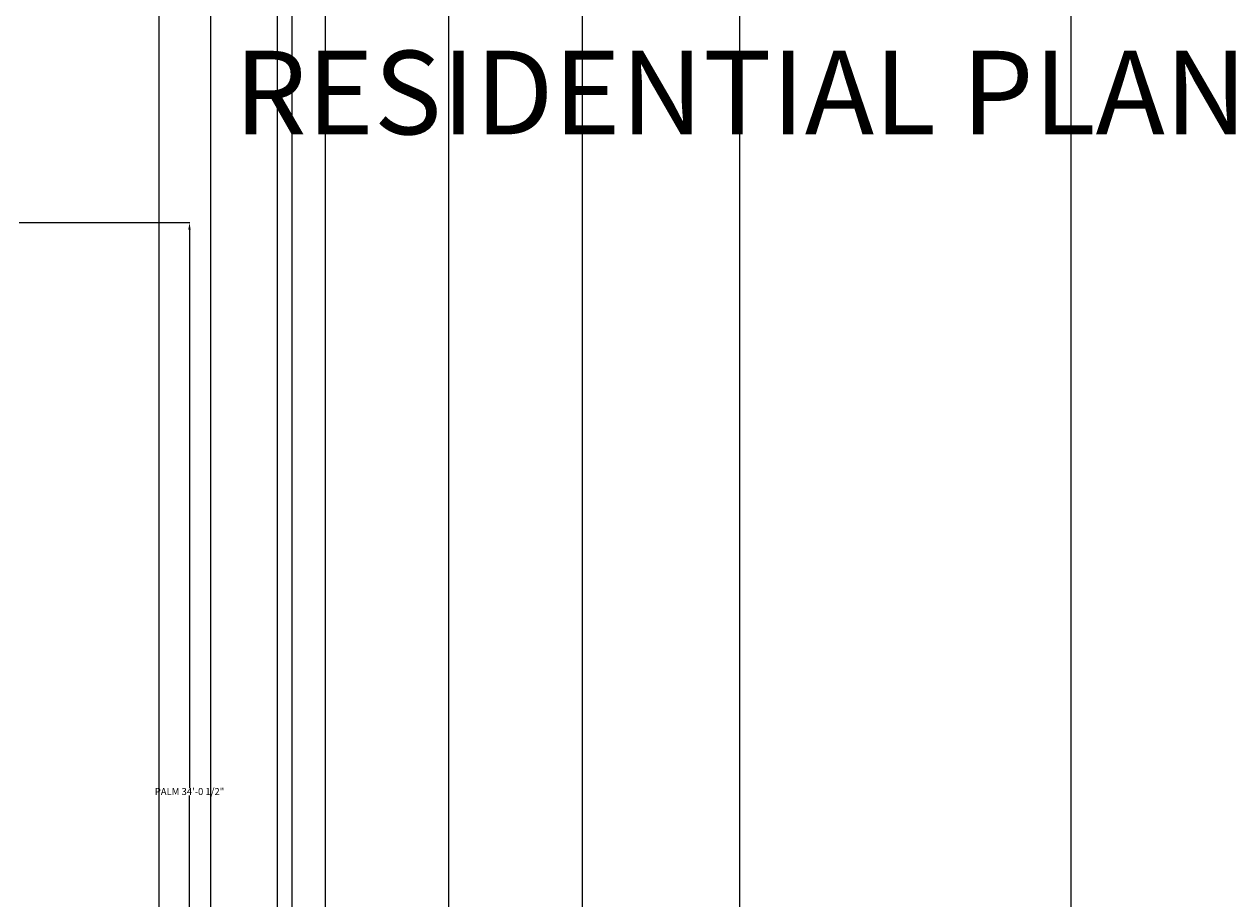
# Model space of a CAD drawing. Units: inches. Extents: x 481 to 2783, y 1975 to 3327.
# Tile 5 of 13: x 1326 to 1761, y 2289 to 2602. Entities that reach past the tile are written whole.
import ezdxf

# ---------------------------------------------------------------- set-up
doc = ezdxf.new("R2010")
doc.units = ezdxf.units.IN
doc.header["$MEASUREMENT"] = 0
doc.layers.add('A-ANNO-DIMS', color=50, linetype='Continuous', lineweight=18)
doc.layers.add('A-ANNO-TEXT', color=50, linetype='Continuous', lineweight=30)
doc.styles.get("Standard").update_dxf_attribs({"font": 'arial.ttf'})
doc.dimstyles.get("Standard").update_dxf_attribs({"dimtxt": 2.5, "dimasz": 2.5, "dimexe": 0.18, "dimexo": 0.0625, "dimgap": 0.09, "dimtad": 0, "dimtih": 1, "dimtoh": 1, "dimzin": 0, "dimdsep": 46, "dimlunit": 3, "dimtxsty": 'Standard', "dimcen": 0.09, "dimadec": 0, "dimazin": 0, "dimtfac": 1, "dimtofl": 0, "dimtmove": 0, "dimatfit": 3, "dimfxl": 1, "dimtolj": 1, "dimtzin": 0, "dimarcsym": 0})

# ---------------------------------------------------------------- blocks, each defined once
blk = doc.blocks.new('*D54')
at = {"layer": 'A-ANNO-DIMS', "color": 0, "lineweight": -2, "transparency": 16777216}
for p, q in [((1324.1, 2531.22), (1385.48, 2531.22)), ((1385.3, 2528.72), (1385.3, 2328.4)), ((1385.3, 2125.32), (1385.3, 2325.64)), ((1324.1, 2122.82), (1385.48, 2122.82))]:
    blk.add_line(p, q, dxfattribs=at)
at = {"layer": 'A-ANNO-DIMS', "color": 0, "transparency": 16777216}
for points in [[(1384.88, 2528.72), (1385.72, 2528.72), (1385.3, 2531.22)], [(1384.88, 2125.32), (1385.72, 2125.32), (1385.3, 2122.82)]]:
    blk.add_solid(points, dxfattribs=at)
at = {"layer": 'Defpoints', "color": 0, "transparency": 16777216}
for p in [(1324.04, 2531.22), (1385.3, 2531.22), (1324.04, 2122.82)]:
    blk.add_point(p, dxfattribs=at)
at = {"layer": 'A-ANNO-DIMS', "color": 0, "transparency": 16777216, "insert": (1385.3, 2327.02), "char_height": 2.5, "attachment_point": 5}
blk.add_mtext('\\A1;PALM 34\'-0 1/2"', dxfattribs=at)
blk = doc.blocks.new('*D76')
at = {"layer": 'A-ANNO-DIMS', "color": 0, "lineweight": -2, "transparency": 16777216}
for p, q in [((1374.44, 2276.88), (1374.44, 2651.23)), ((1376.94, 2651.05), (1377.48, 2651.05)), ((1390.44, 2651.05), (1389.9, 2651.05)), ((1392.94, 2253.88), (1392.94, 2651.23))]:
    blk.add_line(p, q, dxfattribs=at)
at = {"layer": 'A-ANNO-DIMS', "color": 0, "transparency": 16777216}
for points in [[(1376.94, 2651.47), (1376.94, 2650.64), (1374.44, 2651.05)], [(1390.44, 2651.47), (1390.44, 2650.64), (1392.94, 2651.05)]]:
    blk.add_solid(points, dxfattribs=at)
at = {"layer": 'Defpoints', "color": 0, "transparency": 16777216}
for p in [(1392.94, 2651.05), (1374.44, 2276.82), (1392.94, 2253.82)]:
    blk.add_point(p, dxfattribs=at)
at = {"layer": 'A-ANNO-DIMS', "color": 0, "transparency": 16777216, "insert": (1383.69, 2651.05), "char_height": 2.5, "attachment_point": 5}
blk.add_mtext('\\A1;1\'-6 1/2"', dxfattribs=at)
blk = doc.blocks.new('*D77')
at = {"layer": 'A-ANNO-DIMS', "color": 0, "lineweight": -2, "transparency": 16777216}
for p, q in [((1416.94, 2253.88), (1416.94, 2651.23)), ((1419.44, 2651.05), (1441.36, 2651.05)), ((1475.94, 2651.05), (1454.01, 2651.05)), ((1478.44, 2234.88), (1478.44, 2651.23))]:
    blk.add_line(p, q, dxfattribs=at)
at = {"layer": 'A-ANNO-DIMS', "color": 0, "transparency": 16777216}
for points in [[(1419.44, 2651.47), (1419.44, 2650.64), (1416.94, 2651.05)], [(1475.94, 2651.47), (1475.94, 2650.64), (1478.44, 2651.05)]]:
    blk.add_solid(points, dxfattribs=at)
at = {"layer": 'Defpoints', "color": 0, "transparency": 16777216}
for p in [(1478.44, 2651.05), (1416.94, 2253.82), (1478.44, 2234.82)]:
    blk.add_point(p, dxfattribs=at)
at = {"layer": 'A-ANNO-DIMS', "color": 0, "transparency": 16777216, "insert": (1447.69, 2651.05), "char_height": 2.5, "attachment_point": 5}
blk.add_mtext('\\A1;5\'-1 1/2"', dxfattribs=at)
blk = doc.blocks.new('*D78')
at = {"layer": 'A-ANNO-DIMS', "color": 0, "lineweight": -2, "transparency": 16777216}
for p, q in [((1526.44, 2234.88), (1526.44, 2651.23)), ((1528.94, 2651.05), (1548.31, 2651.05)), ((1580.44, 2651.05), (1561.06, 2651.05)), ((1582.94, 2270.88), (1582.94, 2651.23))]:
    blk.add_line(p, q, dxfattribs=at)
at = {"layer": 'A-ANNO-DIMS', "color": 0, "transparency": 16777216}
for points in [[(1528.94, 2651.47), (1528.94, 2650.64), (1526.44, 2651.05)], [(1580.44, 2651.47), (1580.44, 2650.64), (1582.94, 2651.05)]]:
    blk.add_solid(points, dxfattribs=at)
at = {"layer": 'Defpoints', "color": 0, "transparency": 16777216}
for p in [(1582.94, 2651.05), (1582.94, 2270.82), (1526.44, 2234.82)]:
    blk.add_point(p, dxfattribs=at)
at = {"layer": 'A-ANNO-DIMS', "color": 0, "transparency": 16777216, "insert": (1554.69, 2651.05), "char_height": 2.5, "attachment_point": 5}
blk.add_mtext('\\A1;4\'-8 1/2"', dxfattribs=at)
blk = doc.blocks.new('*D79')
at = {"layer": 'A-ANNO-DIMS', "color": 0, "lineweight": -2, "transparency": 16777216}
for p, q in [((1582.94, 2270.88), (1582.94, 2651.23)), ((1585.44, 2651.05), (1638.01, 2651.05)), ((1699.34, 2651.05), (1646.77, 2651.05)), ((1701.84, 2234.88), (1701.84, 2651.23))]:
    blk.add_line(p, q, dxfattribs=at)
at = {"layer": 'A-ANNO-DIMS', "color": 0, "transparency": 16777216}
for points in [[(1585.44, 2651.47), (1585.44, 2650.64), (1582.94, 2651.05)], [(1699.34, 2651.47), (1699.34, 2650.64), (1701.84, 2651.05)]]:
    blk.add_solid(points, dxfattribs=at)
at = {"layer": 'Defpoints', "color": 0, "transparency": 16777216}
for p in [(1701.84, 2651.05), (1582.94, 2270.82), (1701.84, 2234.82)]:
    blk.add_point(p, dxfattribs=at)
at = {"layer": 'A-ANNO-DIMS', "color": 0, "transparency": 16777216, "insert": (1642.39, 2651.05), "char_height": 2.5, "attachment_point": 5}
blk.add_mtext('\\A1;9\'-11"', dxfattribs=at)
blk = doc.blocks.new('*D81')
at = {"layer": 'A-ANNO-DIMS', "color": 0, "lineweight": -2, "transparency": 16777216}
for p, q in [((1422.16, 2270.88), (1422.16, 2651.23)), ((1424.66, 2651.05), (1424.87, 2651.05)), ((1431.66, 2651.05), (1431.46, 2651.05)), ((1434.16, 2270.88), (1434.16, 2651.23))]:
    blk.add_line(p, q, dxfattribs=at)
at = {"layer": 'A-ANNO-DIMS', "color": 0, "transparency": 16777216}
for points in [[(1424.66, 2651.47), (1424.66, 2650.64), (1422.16, 2651.05)], [(1431.66, 2651.47), (1431.66, 2650.64), (1434.16, 2651.05)]]:
    blk.add_solid(points, dxfattribs=at)
at = {"layer": 'Defpoints', "color": 0, "transparency": 16777216}
for p in [(1434.16, 2651.05), (1422.16, 2270.82), (1434.16, 2270.82)]:
    blk.add_point(p, dxfattribs=at)
at = {"layer": 'A-ANNO-DIMS', "color": 0, "transparency": 16777216, "insert": (1428.16, 2651.05), "char_height": 2.5, "attachment_point": 5}
blk.add_mtext('\\A1;1\'-0"', dxfattribs=at)

msp = doc.modelspace()

# ---------------------------------------------------------------- texts
at = {"layer": 'A-ANNO-TEXT', "insert": (1401.392, 2592.901), "char_height": 30, "attachment_point": 1}
msp.add_mtext_dynamic_manual_height_columns('RESIDENTIAL PLAN', width=438.72974, gutter_width=1, heights=[0], dxfattribs=at)

# ---------------------------------------------------------------- dimensions: what is measured, and where the dimension line sits
at = {"layer": 'A-ANNO-DIMS'}
for base, p1, p2, picture, middle in [((1392.938, 2651.053), (1374.438, 2276.821), (1392.938, 2253.821), '*D76', (1383.688, 2651.053)), ((1478.438, 2651.053), (1416.938, 2253.821), (1478.438, 2234.821), '*D77', (1447.688, 2651.053)), ((1582.938, 2651.053), (1526.438, 2234.821), (1582.938, 2270.821), '*D78', (1554.688, 2651.053)), ((1434.162, 2651.053), (1422.162, 2270.821), (1434.162, 2270.821), '*D81', (1428.162, 2651.053)), ((1701.842, 2651.053), (1582.938, 2270.821), (1701.842, 2234.821), '*D79', (1642.39, 2651.053))]:
    dim = msp.add_linear_dim(base=base, p1=p1, p2=p2, dimstyle='Standard', override={"dimdec": 1, "dimlfac": 1, "dimrnd": 0, "dimzin": 1, "dimdsep": 46, "dimlunit": 4, "dimfrac": 2}, dxfattribs=at)
    dim.commit()
    dim.dimension.update_dxf_attribs({"geometry": picture, "text_midpoint": middle})
dim = msp.add_linear_dim(base=(1385.301, 2531.217), p1=(1324.042, 2122.821), p2=(1324.042, 2531.217), angle=90, text='PALM <>', dimstyle='Standard', override={"dimdec": 1, "dimlfac": 1, "dimrnd": 0, "dimzin": 1, "dimdsep": 46, "dimlunit": 4, "dimfrac": 2}, dxfattribs=at)
dim.commit()
dim.dimension.update_dxf_attribs({"geometry": '*D54', "text_midpoint": (1385.301, 2327.019)})

doc.saveas('drawing.dxf')
